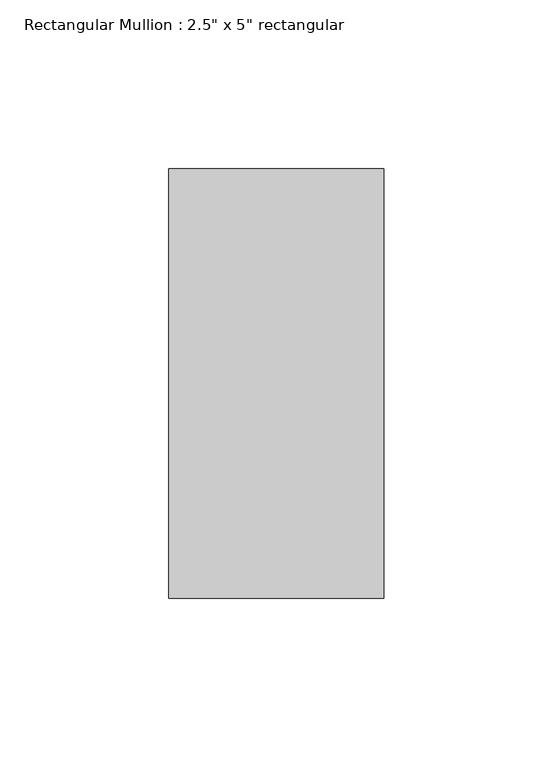
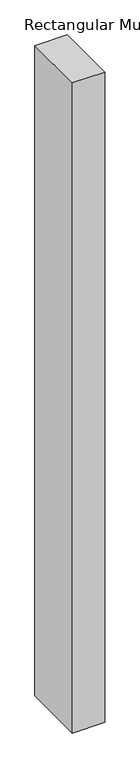
"""IFC4 building model written with IfcOpenShell, lengths in millimetres: member geometry."""

from ifc_helpers import new_model, si_unit, frame, origin, place, context, project, spatial, polyline, outline, extrude, source, transform, mapped, element, save


def member_161f4059(model_context):
    return source(origin(), model_context, "Body", "SweptSolid", [
        extrude(outline(polyline([(31.75, 63.5), (31.75, -63.5), (-31.75, -63.5), (-31.75, 63.5), (31.75, 63.5)])), frame((0.0, 0.0, -1341.9666665), z_axis=(0.0, 0.0, 1.0), x_axis=(1.0, 0.0, 0.0)), (0.0, 0.0, 1.0), 1341.9666665),
    ])


if __name__ == "__main__":
    model = new_model("IFC4")
    model_context = context("Model", 3, world=origin())
    ifc_project = project(units=[si_unit("LENGTHUNIT", "METRE", prefix="MILLI")], contexts=[model_context])
    site = spatial("IfcSite", under=ifc_project)
    building = spatial("IfcBuilding", under=site)
    placement = place(None, origin())
    member_shape = member_161f4059(model_context)
    element("IfcMember", 1, ObjectType="Rectangular Mullion : 2.5\" x 5\" rectangular", at=placement, inside=building, context=model_context, shape_type="MappedRepresentation", body=[
        mapped(member_shape, transform((0.0, 0.0, 0.0), x_axis=(1.0, 0.0, 0.0), y_axis=(0.0, 1.0, 0.0), z_axis=(0.0, 0.0, 1.0))),
    ])
    save(model, "model.ifc")

# Revit data of these elements
# Type "Rectangular Mullion : 2.5\" x 5\" rectangular"
#   built-in parameter 1007304 = 0.416667 (stored number, unit not read)
#   built-in parameter 1007301 = 0.104167 (stored number, unit not read)
#   built-in parameter 1007300 = 0.104167 (stored number, unit not read)
# Element 1 (IfcMember, "Rectangular Mullion : 2.5\" x 5\" rectangular")
#   Materials on its faces: "Aluminum"
# Materials
#   "Aluminum": class "Metal", colour RGB 247 247 247, transparency 0, Description = "Aluminum 6061", Cost = 0
